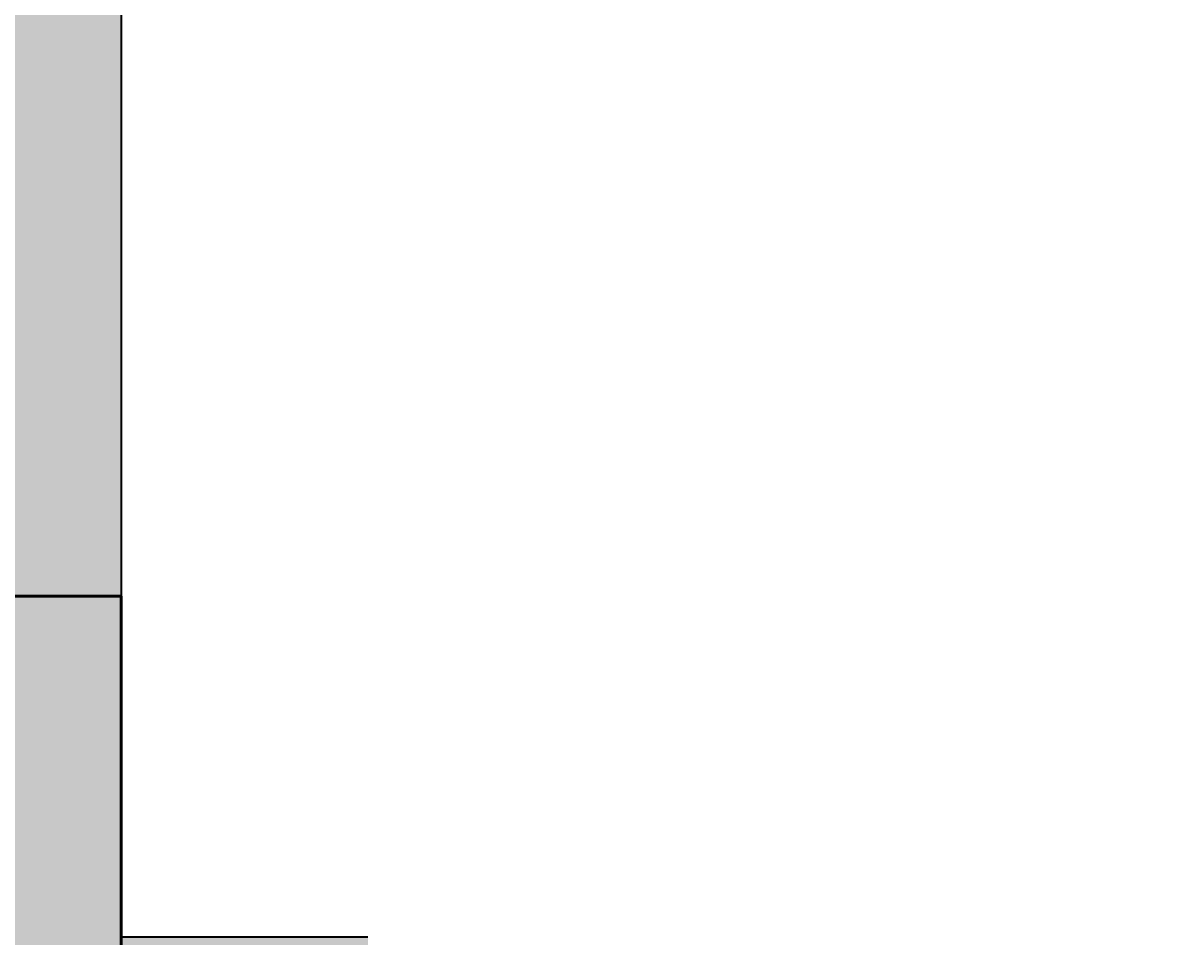
# Model space of a CAD drawing. Units: inches. Extents: x 1998 to 2588, y 1139 to 1977.
# Tile 80 of 134: x 2344 to 2370, y 1481 to 1502. Entities that reach past the tile are written whole.
import ezdxf

# ---------------------------------------------------------------- set-up
doc = ezdxf.new("R2010")
doc.units = ezdxf.units.IN
for name, color, linetype, lineweight in [('A-ANNO-DIMS', 2, 'Continuous', 18), ('A-COLS-PATT', 250, 'Continuous', 13), ('A-WALL-PATT', 252, 'Continuous', 13), ('COLUMN', 10, 'Continuous', 50), ('WALL', 200, 'Continuous', 35)]:
    doc.layers.add(name, color=color, linetype=linetype, lineweight=lineweight)
doc.styles.get("Standard").update_dxf_attribs({"font": 'arial.ttf'})
doc.dimstyles.get("Standard").update_dxf_attribs({"dimtxt": 0.18, "dimasz": 0.18, "dimexe": 0.18, "dimexo": 0.0625, "dimgap": 0.09, "dimtad": 0, "dimtih": 1, "dimtoh": 1, "dimdec": 4, "dimzin": 0, "dimdsep": 46, "dimtxsty": 'Standard', "dimcen": 0.09, "dimadec": 0, "dimazin": 0, "dimtfac": 1, "dimtdec": 4, "dimtofl": 0, "dimtmove": 0, "dimatfit": 3, "dimfxl": 1, "dimtolj": 1, "dimtzin": 0, "dimarcsym": 0})

# ---------------------------------------------------------------- blocks, each defined once
blk = doc.blocks.new('*D43')
at = {"layer": 'A-ANNO-DIMS', "color": 0, "lineweight": -2, "transparency": 16777216}
for p, q in [((2407.973, 1594.67), (2407.973, 1138.602)), ((2345.973, 1588.67), (2345.973, 1138.602)), ((2346.153, 1138.782), (2376.754, 1138.782)), ((2407.793, 1138.782), (2377.191, 1138.782))]:
    blk.add_line(p, q, dxfattribs=at)
at = {"layer": 'A-ANNO-DIMS', "color": 0, "transparency": 16777216}
for points in [[(2346.153, 1138.812), (2346.153, 1138.752), (2345.973, 1138.782)], [(2407.793, 1138.812), (2407.793, 1138.752), (2407.973, 1138.782)]]:
    blk.add_solid(points, dxfattribs=at)
at = {"layer": 'Defpoints', "color": 0, "transparency": 16777216}
for p in [(2407.973, 1594.732), (2345.973, 1588.732), (2407.973, 1138.782)]:
    blk.add_point(p, dxfattribs=at)
at = {"layer": 'A-ANNO-DIMS', "color": 0, "transparency": 16777216, "insert": (2376.973, 1138.782), "char_height": 0.18, "attachment_point": 5}
blk.add_mtext('\\A1;62', dxfattribs=at)

msp = doc.modelspace()

# ---------------------------------------------------------------- hatches: boundary and pattern name
at = {"layer": 'A-COLS-PATT'}
h = msp.add_hatch(color=256, dxfattribs=at)
h.dxf.hatch_style = 1
h.paths.add_polyline_path([(2099.4125, 1888.7324), (2087.9729, 1888.7324), (2087.9729, 1868.3278), (2099.4125, 1868.3278)])
h.paths.add_polyline_path([(2234.4125, 1888.7324), (2222.9729, 1888.7324), (2222.9729, 1868.3278), (2234.4125, 1868.3278)])
h.paths.add_polyline_path([(2341.4729, 1886.637), (2330.0332, 1886.637), (2330.0332, 1866.2324), (2341.4729, 1866.2324)])
h.paths.add_polyline_path([(2507.8006, 1882.7324), (2487.396, 1882.7324), (2487.396, 1871.2927), (2507.8006, 1871.2927)])
h.paths.add_polyline_path([(2510.9729, 1766.672), (2490.5682, 1766.672), (2490.5682, 1755.2324), (2510.9729, 1755.2324)])
h.paths.add_polyline_path([(2345.9729, 1759.7324), (2334.5332, 1759.7324), (2334.5332, 1739.3278), (2345.9729, 1739.3278)])
h.paths.add_polyline_path([(2234.4125, 1774.3318), (2222.9729, 1774.3318), (2222.9729, 1753.9272), (2234.4125, 1753.9272)])
h.paths.add_polyline_path([(2099.4125, 1775.637), (2087.9729, 1775.637), (2087.9729, 1755.2324), (2099.4125, 1755.2324)])
h.paths.add_polyline_path([(2098.0956, 1593.7241), (2077.691, 1593.7241), (2077.691, 1582.2845), (2098.0956, 1582.2845)])
h.paths.add_polyline_path([(2227.4729, 1604.637), (2216.0332, 1604.637), (2216.0332, 1584.2324), (2227.4729, 1584.2324)])
h.paths.add_polyline_path([(2345.9729, 1647.5211), (2334.5332, 1647.5211), (2334.5332, 1627.1165), (2345.9729, 1627.1165)])
h.paths.add_polyline_path([(2522.3775, 1641.2324), (2501.9729, 1641.2324), (2501.9729, 1629.7927), (2522.3775, 1629.7927)])
h.paths.add_polyline_path([(2522.3775, 1480.7324), (2501.9729, 1480.7324), (2501.9729, 1469.2927), (2522.3775, 1469.2927)])
h.paths.add_polyline_path([(2345.9729, 1488.5616), (2334.5332, 1488.5616), (2334.5332, 1468.1569), (2345.9729, 1468.1569)])
h.paths.add_polyline_path([(2234.4125, 1486.137), (2227.4729, 1486.137), (2227.4729, 1465.7324), (2234.4125, 1465.7324)])
h.paths.add_polyline_path([(2227.4729, 1486.137), (2222.9729, 1486.137), (2222.9729, 1465.7324), (2227.4729, 1465.7324)])
h.paths.add_polyline_path([(2108.3775, 1470.2324), (2087.9729, 1470.2324), (2087.9729, 1458.7927), (2108.3775, 1458.7927)])
h.paths.add_polyline_path([(2096.9729, 1365.5012), (2087.9729, 1365.5012), (2087.9729, 1345.0966), (2096.9729, 1345.0966)])
h.paths.add_polyline_path([(2087.9729, 1365.5012), (2085.5332, 1365.5012), (2085.5332, 1345.0966), (2087.9729, 1345.0966)])
h.paths.add_polyline_path([(2234.4125, 1285.137), (2222.9729, 1285.137), (2222.9729, 1264.7324), (2234.4125, 1264.7324)])
h.paths.add_polyline_path([(2345.9729, 1285.137), (2334.5332, 1285.137), (2334.5332, 1264.7324), (2345.9729, 1264.7324)])
h.paths.add_polyline_path([(2503.1458, 1240.172), (2482.7412, 1240.172), (2482.7412, 1228.7324), (2503.1458, 1228.7324)])
h.paths.add_polyline_path([(2510.9729, 1369.172), (2490.5682, 1369.172), (2490.5682, 1357.7324), (2510.9729, 1357.7324)])
at = {"layer": 'A-WALL-PATT'}
h = msp.add_hatch(color=256, dxfattribs=at)
h.dxf.hatch_style = 1
h.paths.add_polyline_path([(2222.9729, 1888.7324), (2099.4125, 1888.7324), (2099.4125, 1879.7324), (2222.9729, 1879.7324)])
h.paths.add_polyline_path([(2096.9729, 1868.3278), (2087.9729, 1868.3278), (2087.9729, 1775.637), (2096.9729, 1775.637)])
h.paths.add_polyline_path([(2227.4729, 1868.3278), (2222.9729, 1868.3278), (2222.9729, 1774.3318), (2227.4729, 1774.3318)])
h.paths.add_polyline_path([(2188.3019, 1759.7324), (2138.6074, 1759.7324), (2099.4125, 1759.7324), (2099.4125, 1755.2324), (2176.9729, 1755.2324), (2188.3019, 1755.2324)])
h.paths.add_polyline_path([(2087.9729, 1759.7324), (2059.4729, 1759.7324), (2059.4729, 1702.7324), (2087.9729, 1702.7324), (2087.9729, 1707.2324), (2063.9729, 1707.2324), (2063.9729, 1755.2324), (2087.9729, 1755.2324)])
h.paths.add_polyline_path([(2096.9729, 1755.2324), (2087.9729, 1755.2324), (2087.9729, 1707.2324), (2096.9729, 1707.2324)])
h.paths.add_polyline_path([(2187.0461, 1707.2324), (2105.9729, 1707.2324), (2096.9729, 1707.2324), (2087.9729, 1707.2324), (2087.9729, 1702.7324), (2105.9729, 1702.7324), (2114.9729, 1702.7324), (2187.0461, 1702.7324)])
h.paths.add_polyline_path([(2181.4729, 1719.2028), (2176.9729, 1719.2028), (2176.9729, 1707.2324), (2181.4729, 1707.2324)])
h.paths.add_polyline_path([(2216.0332, 1588.7324), (2114.9729, 1588.7324), (2105.9729, 1588.7324), (2105.9729, 1584.2324), (2216.0332, 1584.2324)])
h.paths.add_polyline_path([(2077.691, 1588.7324), (2061.4729, 1588.7324), (2061.4729, 1584.2324), (2077.691, 1584.2324)])
h.paths.add_polyline_path([(2105.9729, 1588.7324), (2098.0956, 1588.7324), (2098.0956, 1584.2324), (2105.9729, 1584.2324)])
h.paths.add_polyline_path([(2114.9729, 1596.2642), (2110.1012, 1596.2642), (2105.9729, 1596.2642), (2105.9729, 1588.7324), (2114.9729, 1588.7324)])
h.paths.add_polyline_path([(2114.9729, 1584.2324), (2105.9729, 1584.2324), (2105.9729, 1580.249), (2110.1012, 1580.249), (2114.9729, 1580.249)])
h.paths.add_polyline_path([(2114.9729, 1547.7716), (2110.1012, 1547.7716, -0.0318759), (2105.9729, 1548.035), (2105.9729, 1470.2324), (2108.3775, 1470.2324), (2108.3775, 1465.7324), (2186.2943, 1465.7324), (2186.2943, 1470.2324), (2114.9729, 1470.2324)])
h.paths.add_polyline_path([(2227.4729, 1584.2324), (2222.9729, 1584.2324), (2222.9729, 1486.137), (2227.4729, 1486.137)])
h.paths.add_polyline_path([(2295.4138, 1593.2324), (2227.4729, 1593.2324), (2227.4729, 1588.7324), (2295.4138, 1588.7324), (2295.4138, 1591.8729)])
h.paths.add_polyline_path([(2345.9729, 1627.1165), (2341.4729, 1627.1165), (2341.4729, 1593.2324), (2337.2869, 1593.2324), (2337.2869, 1591.8729), (2337.2869, 1588.7324), (2345.9729, 1588.7324)])
h.paths.add_polyline_path([(2291.9729, 1588.7324), (2287.4729, 1588.7324), (2287.4729, 1522.7324), (2291.9729, 1522.7324)])
h.paths.add_polyline_path([(2291.9729, 1522.7324), (2287.4729, 1522.7324), (2227.4729, 1522.7324), (2227.4729, 1518.2324), (2291.9729, 1518.2324)])
h.paths.add_polyline_path([(2295.7347, 1519.5919), (2295.7347, 1522.7324), (2291.9729, 1522.7324), (2291.9729, 1518.2324), (2295.7347, 1518.2324)])
h.paths.add_polyline_path([(2345.9729, 1522.7324), (2337.6078, 1522.7324), (2337.6078, 1519.5919), (2337.6078, 1518.2324), (2341.4729, 1518.2324), (2341.4729, 1488.5616), (2345.9729, 1488.5616)])
h.paths.add_polyline_path([(2345.9729, 1468.1569), (2341.4729, 1468.1569), (2341.4729, 1374.2324), (2227.4729, 1374.2324), (2227.4729, 1369.7324), (2345.9729, 1369.7324)])
h.paths.add_polyline_path([(2345.9729, 1369.7324), (2341.4729, 1369.7324), (2341.4729, 1362.2324), (2345.9729, 1362.2324)])
h.paths.add_polyline_path([(2345.9729, 1317.7324), (2345.9729, 1322.2324), (2341.4729, 1322.2324), (2341.4729, 1285.137), (2345.9729, 1285.137)], flags=17)
h.paths.add_polyline_path([(2356.2096, 1322.2324), (2345.9729, 1322.2324), (2345.9729, 1317.7324), (2356.2096, 1317.7324), (2356.2096, 1319.3088)], flags=17)
h.paths.add_polyline_path([(2393.9729, 1322.2324), (2375.6999, 1322.2324), (2375.6999, 1319.3088, -0.0202458), (2375.636, 1317.7324), (2393.9729, 1317.7324)], flags=17)
h.paths.add_polyline_path([(2398.4729, 1322.2324), (2393.9729, 1322.2324), (2393.9729, 1317.7324), (2393.9729, 1237.7324), (2345.9729, 1237.7324), (2345.9729, 1264.7324), (2341.4729, 1264.7324), (2341.4729, 1228.7324), (2393.9729, 1228.7324), (2482.7412, 1228.7324), (2482.7412, 1237.7324), (2398.4729, 1237.7324), (2398.4729, 1297.1029)])
h.paths.add_polyline_path([(2398.4729, 1362.2324), (2393.9729, 1362.2324), (2393.9729, 1357.7324), (2398.4729, 1357.7324)])
h.paths.add_polyline_path([(2345.9729, 1329.7549), (2341.4729, 1329.7549), (2341.4729, 1322.2324), (2345.9729, 1322.2324)])
h = msp.add_hatch(color=256, dxfattribs=at)
h.dxf.hatch_style = 1
h.paths.add_polyline_path([(2527.4729, 1362.2324), (2510.9729, 1362.2324), (2510.9729, 1357.7324), (2518.4729, 1357.7324), (2518.4729, 1237.7324), (2503.1458, 1237.7324), (2503.1458, 1228.7324), (2527.4729, 1228.7324)])
h.paths.add_polyline_path([(2490.5682, 1362.2324), (2398.4729, 1362.2324), (2398.4729, 1357.7324), (2490.5682, 1357.7324)])
h.paths.add_polyline_path([(2224.9729, 1264.7324), (2222.9729, 1264.7324), (2222.9729, 1232.4125), (2341.4729, 1232.4125), (2341.4729, 1234.4125), (2224.9729, 1234.4125)])
h.paths.add_polyline_path([(2334.5332, 1273.7324), (2264.7638, 1273.7324), (2264.7638, 1269.5611, -0.043659), (2264.3413, 1264.7324), (2334.5332, 1264.7324)])
h.paths.add_polyline_path([(2236.9551, 1273.7324), (2234.4125, 1273.7324), (2234.4125, 1264.7324), (2236.9551, 1264.7324), (2236.9551, 1269.5611)])
h.paths.add_polyline_path([(2222.9729, 1293.2324), (2096.9729, 1293.2324), (2096.9729, 1345.0966), (2087.9729, 1345.0966), (2087.9729, 1284.2324), (2222.9729, 1284.2324), (2222.9729, 1285.137)])
h.paths.add_polyline_path([(2096.9729, 1458.7927), (2087.9729, 1458.7927), (2087.9729, 1417.7324), (2087.9729, 1413.2324), (2096.9729, 1413.2324), (2096.9729, 1417.7324)])
h.paths.add_polyline_path([(2096.9729, 1413.2324), (2087.9729, 1413.2324), (2087.9729, 1365.5012), (2096.9729, 1365.5012), (2096.9729, 1369.3358)])
h.paths.add_polyline_path([(2186.2943, 1417.7324), (2138.6074, 1417.7324), (2096.9729, 1417.7324), (2096.9729, 1413.2324), (2138.6074, 1413.2324), (2186.2943, 1413.2324)])
h.paths.add_polyline_path([(2181.4729, 1465.7324), (2176.9729, 1465.7324), (2176.9729, 1451.6434), (2181.4729, 1451.6434)])
h.paths.add_polyline_path([(2181.4729, 1422.1664), (2176.9729, 1422.1664), (2176.9729, 1417.7324), (2181.4729, 1417.7324)])
h.paths.add_polyline_path([(2063.9729, 1465.7324), (2087.9729, 1465.7324), (2087.9729, 1470.2324), (2059.4729, 1470.2324), (2059.4729, 1413.2324), (2087.9729, 1413.2324), (2087.9729, 1417.7324), (2063.9729, 1417.7324)])
h.paths.add_polyline_path([(2181.4729, 1755.2324), (2176.9729, 1755.2324), (2176.9729, 1748.6798), (2177.0513, 1748.6798), (2181.4729, 1748.6798)])
h.paths.add_polyline_path([(2227.4729, 1707.2324), (2220.4647, 1707.2324), (2220.4647, 1702.7324), (2222.9729, 1702.7324), (2222.9729, 1604.637), (2227.4729, 1604.637)])
h.paths.add_polyline_path([(2114.9729, 1702.7324), (2105.9729, 1702.7324), (2105.9729, 1628.4781, -0.0318759), (2110.1012, 1628.7416), (2114.9729, 1628.7416)])
h.paths.add_polyline_path([(2345.9729, 1739.3278), (2341.4729, 1739.3278), (2341.4729, 1647.5211), (2345.9729, 1647.5211)])
h.paths.add_polyline_path([(2350.6273, 1641.2324), (2345.9729, 1641.2324), (2345.9729, 1636.7324), (2350.6273, 1636.7324), (2350.6273, 1639.8729)])
h.paths.add_polyline_path([(2501.9729, 1641.2324), (2407.9729, 1641.2324), (2392.5005, 1641.2324), (2392.5005, 1639.8729), (2392.5005, 1636.7324), (2501.9729, 1636.7324)])
h.paths.add_polyline_path([(2510.9729, 1755.2324), (2501.9729, 1755.2324), (2501.9729, 1641.2324), (2510.9729, 1641.2324)])
h.paths.add_polyline_path([(2549.1786, 1641.2324), (2522.3775, 1641.2324), (2522.3775, 1636.7324), (2540.1786, 1636.7324), (2540.1786, 1480.7324), (2522.3775, 1480.7324), (2522.3775, 1476.2324), (2549.1786, 1476.2324)])
h.paths.add_polyline_path([(2498.1786, 1594.7324), (2407.9729, 1594.7324), (2407.9729, 1585.7324), (2416.9729, 1585.7324), (2489.1786, 1585.7324), (2489.1786, 1531.7324), (2416.9729, 1531.7324), (2407.9729, 1531.7324), (2407.9729, 1522.7324), (2498.1786, 1522.7324)])
h.paths.add_polyline_path([(2351.6437, 1480.7324), (2345.9729, 1480.7324), (2345.9729, 1476.2324), (2351.6437, 1476.2324), (2351.6437, 1477.5919)])
h.paths.add_polyline_path([(2501.9729, 1480.7324), (2498.1786, 1480.7324), (2407.9729, 1480.7324), (2393.5168, 1480.7324), (2393.5168, 1477.5919), (2393.5168, 1476.2324), (2501.9729, 1476.2324)])

# ---------------------------------------------------------------- linework, layer by layer
at = {"layer": 'COLUMN'}
msp.add_lwpolyline([(2334.5332, 1488.5616), (2345.9729, 1488.5616), (2345.9729, 1468.1569), (2334.5332, 1468.1569)], close=True, dxfattribs=at)
at = {"layer": 'WALL'}
for p, q in [((2345.9729, 1522.7324), (2345.9729, 1369.7324)), ((2345.9729, 1522.7324), (2345.9729, 1480.7324)), ((2345.9729, 1480.7324), (2351.6437, 1480.7324))]:
    msp.add_line(p, q, dxfattribs=at)

# ---------------------------------------------------------------- dimensions: what is measured, and where the dimension line sits
at = {"layer": 'A-ANNO-DIMS'}
dim = msp.add_linear_dim(base=(2407.9729, 1138.7824), p1=(2345.9729, 1588.7324), p2=(2407.9729, 1594.7324), dimstyle='Standard', override={"dimdec": 0, "dimlfac": 1, "dimrnd": 0, "dimzin": 0, "dimdsep": 46, "dimlunit": 2}, dxfattribs=at)
dim.commit()
dim.dimension.update_dxf_attribs({"geometry": '*D43', "text_midpoint": (2376.9729, 1138.7824)})

doc.saveas('drawing.dxf')
